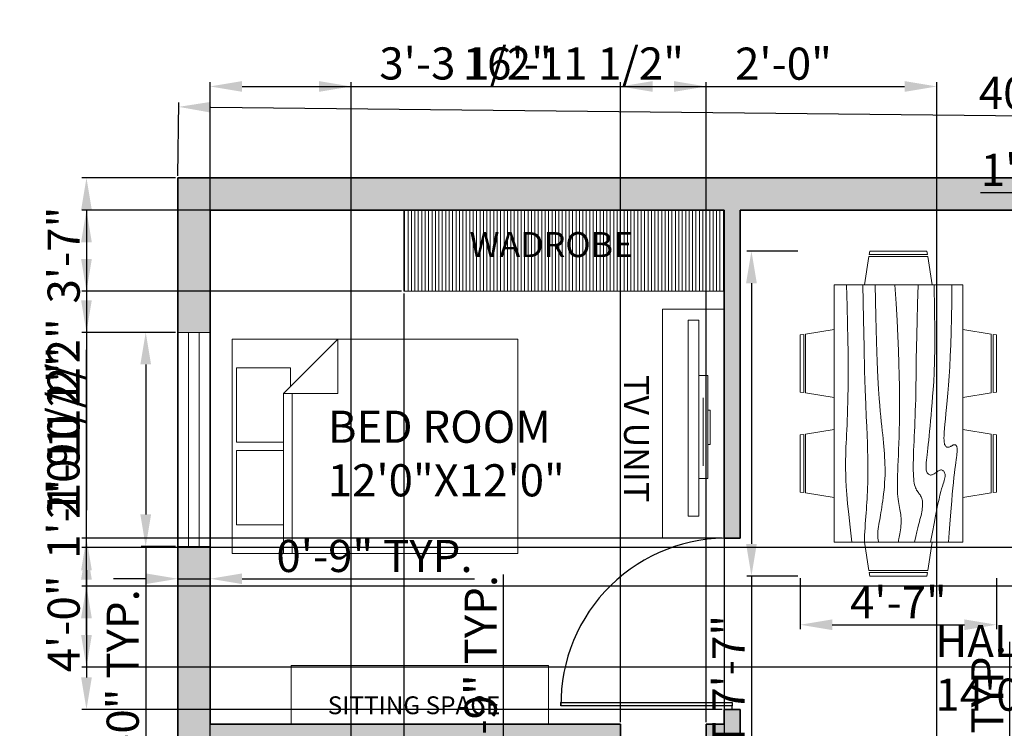
# Model space of a CAD drawing. Units: inches. Extents: x 33024 to 33675, y 11501 to 11939.
# Tile 2 of 3: x 33024 to 33299, y 11741 to 11939. Entities that reach past the tile are written whole.
import ezdxf

# ---------------------------------------------------------------- set-up
doc = ezdxf.new("R2010")
doc.units = ezdxf.units.IN
for name, color, linetype, lineweight in [('A-ANNO-DIMS', 2, 'Continuous', 18), ('A-ANNO-TEXT', 7, 'Continuous', 18), ('A-AREA-IDEN', 7, 'Continuous', 18), ('A-DOOR', 4, 'Continuous', 25), ('A-FURN', 8, 'Continuous', 18), ('A-FURN-FIXD', 8, 'Continuous', 18), ('A-FURN-PATT', 252, 'Continuous', 9), ('A-GLAZ', 4, 'Continuous', 18), ('A-WALL', 7, 'Continuous', 35)]:
    doc.layers.add(name, color=color, linetype=linetype, lineweight=lineweight)
doc.layers.add('A-WALL-PATT', color=242, linetype='Continuous', lineweight=13, true_color=0xcd2027)
doc.styles.get("Standard").update_dxf_attribs({"font": 'arial.ttf'})
doc.dimstyles.new('ISO-25', dxfattribs={"dimtxt": 9, "dimasz": 9, "dimexe": 1.25, "dimexo": 0.625, "dimtad": 1, "dimdec": 1, "dimrnd": 9, "dimlunit": 3, "dimtxsty": 'Standard', "dimcen": 2.5, "dimadec": 0, "dimazin": 0, "dimtfac": 1, "dimtdec": 1, "dimtmove": 0, "dimatfit": 3, "dimfxl": 1, "dimarcsym": 0})

# ---------------------------------------------------------------- blocks, each defined once
blk = doc.blocks.new('Bed - Queen')
for p, q in [((0, -80.00003), (0, 0)), ((0, 0), (59.99999, 0)), ((59.99999, 0), (59.99999, -80.00003)), ((7.99999, -1.2), (28.79998, -1.2)), ((7.99999, -14.4), (7.99999, -1.2)), ((28.79998, -1.2), (28.79998, -14.4)), ((31.19999, -1.2), (51.99999, -1.2)), ((31.19999, -14.4), (31.19999, -1.2)), ((51.99999, -1.2), (51.99999, -16.4)), ((0, -14.4), (44.8, -14.4)), ((59.99999, -29.6), (44.8, -14.4)), ((44.8, -14.4), (44.8, -29.6)), ((51.99999, -16.4), (46.79936, -16.4)), ((44.8, -16.8), (0, -16.8)), ((44.8, -29.6), (59.99999, -29.6)), ((59.99999, -80.00003), (0, -80.00003))]:
    blk.add_line(p, q)
blk = doc.blocks.new('Dining Set - 36 x 72 in.')
for p, q in [((-22.2343, 26.00059), (-23.4847, 17.99762)), ((-22.2304, 26), (-5.7608, 26)), ((-22, 27.5), (-22.1562, 26.50042)), ((-5.8416, 26.5), (-22.1534, 26.5)), ((-22, 27.5), (-6, 27.5)), ((-5.8437, 26.49966), (-6, 27.5)), ((-4.5152, 17.99762), (-5.7655, 25.99926)), ((5.7657, 26.00059), (4.5153, 17.99762)), ((5.7696, 26), (22.2392, 26)), ((6, 27.5), (5.8438, 26.50042)), ((22.1584, 26.5), (5.8466, 26.5)), ((6, 27.5), (22, 27.5)), ((22.1563, 26.49966), (22, 27.5)), ((23.4848, 17.99762), (22.2345, 25.99926)), ((36, 18), (-36, 18)), ((-36, 18), (-36, -18)), ((36, -18), (36, 18)), ((-44.0006, 8.23428), (-35.9976, 9.48474)), ((44.0006, 8.23428), (35.9976, 9.48474)), ((-45.5, 8), (-44.5004, 8.15617)), ((-45.5, 8), (-45.5, -8)), ((-44.5, -8.15843), (-44.5, 8.15338)), ((-44, 8.23041), (-44, -8.23915)), ((44, 8.23041), (44, -8.23915)), ((44.5, -8.15843), (44.5, 8.15338)), ((45.5, 8), (44.5005, 8.15617)), ((45.5, 8), (45.5, -8)), ((-44.4997, -8.15631), (-45.5, -8)), ((-35.9976, -9.48476), (-43.9993, -8.2345)), ((35.9976, -9.48476), (43.9993, -8.2345)), ((44.4997, -8.15631), (45.5, -8)), ((-36, -18), (36, -18)), ((-22.2343, -26.0006), (-23.4847, -17.99762)), ((-4.5152, -17.99762), (-5.7655, -25.99928)), ((5.7657, -26.0006), (4.5153, -17.99762)), ((23.4848, -17.99762), (22.2345, -25.99928)), ((-22.2304, -26), (-5.7608, -26)), ((-22, -27.5), (-22.1562, -26.50044)), ((-5.8416, -26.5), (-22.1534, -26.5)), ((-22, -27.5), (-6, -27.5)), ((-5.8437, -26.49967), (-6, -27.5)), ((5.7696, -26), (22.2392, -26)), ((6, -27.5), (5.8438, -26.50044)), ((22.1584, -26.5), (5.8466, -26.5)), ((6, -27.5), (22, -27.5)), ((22.1563, -26.49967), (22, -27.5))]:
    blk.add_line(p, q)
for points in [[(-36, 15), (-31.1772, 14.97754), (-26.8079, 14.91406), (-22.8538, 14.81543), (-19.276, 14.6875), (-16.0362, 14.53613), (-13.0957, 14.36718), (-10.4159, 14.18652), (-7.9583, 14), (-5.6904, 13.81315), (-3.6035, 13.63021), (-1.6954, 13.45508), (0.0365, 13.29166), (1.5945, 13.14388), (2.9811, 13.01562), (4.1988, 12.9108), (5.25, 12.83333), (6.1393, 12.78613), (6.8802, 12.76823), (7.4883, 12.77767), (7.9792, 12.8125), (8.3685, 12.87077), (8.6719, 12.95052), (8.9049, 13.0498), (9.0833, 13.16666), (9.2205, 13.29899), (9.3216, 13.44401), (9.3895, 13.59879), (9.4271, 13.76041), (9.4373, 13.92594), (9.4232, 14.09245), (9.3875, 14.257), (9.3333, 14.41666), (9.2638, 14.56917), (9.1836, 14.71484), (9.0975, 14.85465), (9.0104, 14.98958), (8.9272, 15.1206), (8.8529, 15.2487), (8.7922, 15.37483), (8.75, 15.5), (8.7305, 15.62467), (8.7344, 15.74739), (8.7617, 15.86621), (8.8125, 15.97916), (8.8867, 16.08431), (8.9844, 16.17968), (9.1055, 16.26334), (9.25, 16.33333), (9.4189, 16.38802), (9.6172, 16.42708), (9.8506, 16.45052), (10.125, 16.45833), (10.4463, 16.45052), (10.8203, 16.42708), (11.2529, 16.38802), (11.75, 16.33333), (12.3184, 16.26318), (12.9694, 16.17838), (13.7151, 16.07991), (14.5677, 15.96875), (15.5395, 15.84586), (16.6426, 15.71224), (17.8893, 15.56884), (19.2917, 15.41666), (20.859, 15.25667), (22.5879, 15.08984), (24.4721, 14.91715), (26.5052, 14.73958), (28.6809, 14.5581), (30.9929, 14.3737), (33.4347, 14.18733), (36, 14)], [(-36, 10), (-28.9766, 10.14274), (-23.1725, 10.20442), (-18.4241, 10.19775), (-14.5677, 10.13541), (-11.4399, 10.03011), (-8.877, 9.89453), (-6.7154, 9.74137), (-4.7917, 9.58333), (-2.9698, 9.43082), (-1.2246, 9.28515), (0.4415, 9.14534), (2.026, 9.01041), (3.5266, 8.87939), (4.9408, 8.7513), (6.266, 8.62516), (7.5, 8.5), (8.6411, 8.37549), (9.6914, 8.2539), (10.6538, 8.13818), (11.5312, 8.03125), (12.3267, 7.93603), (13.043, 7.85547), (13.6831, 7.79248), (14.25, 7.75), (14.7471, 7.7303), (15.1797, 7.73307), (15.5537, 7.75732), (15.875, 7.80208), (16.1494, 7.86637), (16.3828, 7.94922), (16.5811, 8.04964), (16.75, 8.16666), (16.8944, 8.29915), (17.0143, 8.44531), (17.1089, 8.60319), (17.1771, 8.77083), (17.218, 8.94629), (17.2305, 9.1276), (17.2137, 9.31282), (17.1667, 9.5), (17.0895, 9.6875), (16.987, 9.875), (16.8649, 10.0625), (16.7292, 10.25), (16.5856, 10.4375), (16.4401, 10.625), (16.2985, 10.8125), (16.1667, 11), (16.05, 11.18733), (15.9518, 11.3737), (15.8752, 11.5581), (15.8229, 11.73958), (15.798, 11.91715), (15.8034, 12.08984), (15.842, 12.25667), (15.9167, 12.41666), (16.0295, 12.56836), (16.1784, 12.70833), (16.3605, 12.83268), (16.5729, 12.9375), (16.8127, 13.01888), (17.0768, 13.07291), (17.3625, 13.0957), (17.6667, 13.08333), (17.9894, 13.03312), (18.3418, 12.94726), (18.7382, 12.82918), (19.1927, 12.68229), (19.7195, 12.51001), (20.3327, 12.31575), (21.0465, 12.10294), (21.875, 11.875), (22.8357, 11.63354), (23.959, 11.37304), (25.2786, 11.08618), (26.8282, 10.76562), (28.6414, 10.40405), (30.752, 9.99414), (33.1936, 9.52856), (36, 9)], [(-36, 5.5), (-30.7157, 5.3348), (-26.069, 5.20963), (-21.9946, 5.11767), (-18.4271, 5.05208), (-15.3009, 5.00602), (-12.5508, 4.97265), (-10.1112, 4.94515), (-7.9167, 4.91666), (-5.909, 4.88167), (-4.0586, 4.83984), (-2.3429, 4.79215), (-0.7396, 4.73958), (0.7739, 4.6831), (2.22, 4.6237), (3.6213, 4.56233), (5, 4.5), (6.373, 4.43782), (7.7344, 4.3776), (9.0723, 4.32129), (10.375, 4.27083), (11.6309, 4.22819), (12.8281, 4.19531), (13.9551, 4.17415), (15, 4.16666), (15.954, 4.17448), (16.819, 4.19791), (17.6001, 4.23698), (18.3021, 4.29166), (18.9299, 4.36198), (19.4883, 4.44791), (19.9823, 4.54948), (20.4167, 4.66666), (20.7969, 4.79899), (21.1302, 4.94401), (21.4245, 5.09879), (21.6875, 5.26041), (21.9271, 5.42594), (22.1511, 5.59245), (22.3672, 5.757), (22.5834, 5.91666), (22.8065, 6.06868), (23.0404, 6.21093), (23.2879, 6.34147), (23.5521, 6.45833), (23.8358, 6.55957), (24.142, 6.64323), (24.4735, 6.70735), (24.8334, 6.75), (25.2235, 6.76969), (25.642, 6.76692), (26.0858, 6.74267), (26.5521, 6.69791), (27.0379, 6.63362), (27.5404, 6.55078), (28.0565, 6.45036), (28.5834, 6.33333), (29.1242, 6.19987), (29.7071, 6.04687), (30.3661, 5.87044), (31.1354, 5.66666), (32.0493, 5.43164), (33.142, 5.16146), (34.4475, 4.85221), (36, 4.5)], [(-36, -1), (-30.7915, -0.6591), (-26.0195, -0.38216), (-21.6519, -0.16284), (-17.6563, 0.00521), (-14.0005, 0.12833), (-10.6523, 0.21289), (-7.5796, 0.26522), (-4.75, 0.29166), (-2.134, 0.29793), (0.2878, 0.28711), (2.5317, 0.26163), (4.6146, 0.22396), (6.5529, 0.17651), (8.3633, 0.12174), (10.0623, 0.06209), (11.6667, 0), (13.1899, -0.06201), (14.6341, -0.1211), (15.9982, -0.17432), (17.2813, -0.21875), (18.4823, -0.25147), (19.6003, -0.26953), (20.6343, -0.27002), (21.5834, -0.25), (22.4481, -0.20768), (23.2357, -0.14584), (23.9549, -0.06836), (24.6146, 0.02083), (25.2235, 0.11784), (25.7904, 0.21875), (26.3241, 0.31966), (26.8334, 0.41666), (27.3265, 0.50618), (27.8099, 0.58593), (28.2894, 0.65397), (28.7709, 0.70833), (29.2601, 0.74707), (29.763, 0.76823), (30.2855, 0.76985), (30.8334, 0.75), (31.4088, 0.70784), (31.9994, 0.64713), (32.589, 0.57275), (33.1615, 0.48958), (33.7008, 0.4025), (34.1908, 0.3164), (34.6153, 0.23616), (34.9584, 0.16666), (35.2099, 0.11165), (35.3848, 0.07031), (35.504, 0.04069), (35.5886, 0.02083), (35.6594, 0.00879), (35.7377, 0.0026), (35.8442, 0.00032), (36, 0)], [(-36, -6.5), (-27.1843, -6.31267), (-20.084, -6.1263), (-14.469, -5.9419), (-10.1094, -5.76042), (-6.7752, -5.58285), (-4.2363, -5.41016), (-2.2629, -5.24333), (-0.625, -5.08334), (0.8708, -4.93099), (2.2715, -4.78646), (3.5872, -4.64974), (4.8281, -4.52084), (6.0046, -4.39974), (7.127, -4.28646), (8.2053, -4.18099), (9.25, -4.08334), (10.2705, -3.99382), (11.2734, -3.91407), (12.2647, -3.84603), (13.25, -3.79167), (14.2354, -3.75293), (15.2266, -3.73177), (16.2295, -3.73015), (17.25, -3.75), (18.2912, -3.79248), (19.3451, -3.85547), (20.4009, -3.93604), (21.4479, -4.03125), (22.4754, -4.13819), (23.4727, -4.25391), (24.4289, -4.37549), (25.3334, -4.5), (26.1785, -4.62492), (26.9694, -4.74935), (27.7145, -4.87281), (28.4219, -4.99479), (29.1, -5.11483), (29.7572, -5.23242), (30.4016, -5.34709), (31.0417, -5.45834), (31.6837, -5.56437), (32.3262, -5.65821), (32.9658, -5.73153), (33.599, -5.77604), (34.2224, -5.78345), (34.8327, -5.74545), (35.4264, -5.65373), (36, -5.5)], [(-36, -10), (-26.4022, -9.81299), (-18.4675, -9.62891), (-11.9839, -9.45069), (-6.7396, -9.28125), (-2.5226, -9.12354), (0.8789, -8.98047), (3.6769, -8.85498), (6.0833, -8.75), (8.2767, -8.66765), (10.3021, -8.60677), (12.1712, -8.56543), (13.8958, -8.54167), (15.4876, -8.53353), (16.9583, -8.53907), (18.3197, -8.55632), (19.5834, -8.58334), (20.7616, -8.61841), (21.8685, -8.66081), (22.9188, -8.71004), (23.9271, -8.76563), (24.9081, -8.82707), (25.8763, -8.89388), (26.8465, -8.96558), (27.8334, -9.04167), (28.8474, -9.12118), (29.8828, -9.20117), (30.93, -9.27824), (31.9792, -9.34896), (33.0205, -9.40991), (34.0443, -9.45768), (35.0407, -9.48885), (36, -9.5)], [(-36, -14.5), (-30.0881, -14.33513), (-25.0332, -14.21224), (-20.7312, -14.12647), (-17.0781, -14.07292), (-13.97, -14.04671), (-11.3027, -14.04297), (-8.9724, -14.05681), (-6.875, -14.08334), (-4.9224, -14.11833), (-3.0905, -14.16016), (-1.3709, -14.20785), (0.2448, -14.26042), (1.7647, -14.3169), (3.1973, -14.3763), (4.5507, -14.43767), (5.8333, -14.5), (7.0554, -14.5621), (8.235, -14.62175), (9.3922, -14.67652), (10.5469, -14.72396), (11.7192, -14.76164), (12.929, -14.78711), (14.1965, -14.79794), (15.5417, -14.79167), (16.9933, -14.76424), (18.6152, -14.70508), (20.4804, -14.60197), (22.6615, -14.44271), (25.2312, -14.21509), (28.2624, -13.9069), (31.8277, -13.50594), (36, -13)]]:
    blk.add_lwpolyline(points)
blk = doc.blocks.new('*D8')
at = {"layer": 'A-ANNO-DIMS', "color": 0, "lineweight": -2, "transparency": 16777216}
for p, q in [((33068.04, 11895.8), (33068.26, 11916.32)), ((33077.25, 11914.97), (33541.21, 11909.99)), ((33550.01, 11890.62), (33550.23, 11911.14))]:
    blk.add_line(p, q, dxfattribs=at)
at = {"layer": 'A-ANNO-DIMS', "color": 0, "transparency": 16777216}
for points in [[(33077.26, 11916.47), (33077.23, 11913.47), (33068.25, 11915.07)], [(33541.23, 11911.49), (33541.2, 11908.49), (33550.21, 11909.89)]]:
    blk.add_solid(points, dxfattribs=at)
at = {"layer": 'Defpoints', "color": 0, "transparency": 16777216}
for p in [(33550.21, 11909.89), (33068.03, 11895.18), (33550, 11890)]:
    blk.add_point(p, dxfattribs=at)
at = {"layer": 'A-ANNO-DIMS', "color": 0, "transparency": 16777216, "insert": (33309.29, 11917.7), "char_height": 9, "attachment_point": 5, "rotation": 359.3847}
blk.add_mtext('40\'-6"', dxfattribs=at)
blk = doc.blocks.new('TV-CONSOLE-64')
for p, q in [((-17.33, 64.14), (-17.33, 0)), ((-7.13, 45.53), (-7.13, 45.53)), ((-7.13, 45.53), (-4.58, 45.53)), ((-4.58, 45.53), (-4.58, 16.72)), ((-5.92, 39.3), (-5.92, 20.26)), ((-4.58, 35.87), (-3.95, 35.87)), ((-3.95, 35.87), (-3.95, 26.18)), ((-3.95, 26.18), (-4.58, 26.18)), ((-4.58, 16.72), (-7.13, 16.72))]:
    blk.add_line(p, q)
blk.add_lwpolyline([(-17.33, 64.14), (0, 64.14), (0, 0), (-17.33, 0)])
blk.add_lwpolyline([(-10.08, 61), (-7.13, 61), (-7.13, 6.14), (-10.08, 6.14)], close=True)
blk = doc.blocks.new('WIN-60X9')
for p, q in [((0, 9), (0, 0)), ((60, 9), (60, 0)), ((60, 6), (0, 6)), ((60, 3), (0, 3))]:
    blk.add_line(p, q)
blk = doc.blocks.new('*D12')
at = {"layer": 'A-ANNO-DIMS', "color": 0, "lineweight": -2, "transparency": 16777216}
for p, q in [((33067.41, 11851.93), (33057.78, 11851.93)), ((33059.03, 11842.93), (33059.03, 11800.93)), ((33067.41, 11791.93), (33057.78, 11791.93)), ((33059.03, 11791.93), (33059.03, 11667.8))]:
    blk.add_line(p, q, dxfattribs=at)
at = {"layer": 'A-ANNO-DIMS', "color": 0, "transparency": 16777216}
for points in [[(33057.53, 11842.93), (33060.53, 11842.93), (33059.03, 11851.93)], [(33057.53, 11800.93), (33060.53, 11800.93), (33059.03, 11791.93)]]:
    blk.add_solid(points, dxfattribs=at)
at = {"layer": 'Defpoints', "color": 0, "transparency": 16777216}
for p in [(33068.03, 11851.93), (33059.03, 11791.93), (33068.03, 11791.93)]:
    blk.add_point(p, dxfattribs=at)
at = {"layer": 'A-ANNO-DIMS', "color": 0, "transparency": 16777216, "insert": (33053.75, 11725.37), "char_height": 9, "attachment_point": 5, "rotation": 90}
blk.add_mtext('WINDOW 5\'-0" TYP.', dxfattribs=at)
blk = doc.blocks.new('*D13')
at = {"layer": 'A-ANNO-DIMS', "color": 0, "lineweight": -2, "transparency": 16777216}
for p, q in [((33068.03, 11791.31), (33068.03, 11781.68)), ((33077.03, 11791.31), (33077.03, 11781.68)), ((33059.03, 11782.93), (33050.03, 11782.93)), ((33068.03, 11782.93), (33077.03, 11782.93)), ((33086.03, 11782.93), (33151.14, 11782.93))]:
    blk.add_line(p, q, dxfattribs=at)
at = {"layer": 'A-ANNO-DIMS', "color": 0, "transparency": 16777216}
for points in [[(33059.03, 11784.43), (33059.03, 11781.43), (33068.03, 11782.93)], [(33086.03, 11784.43), (33086.03, 11781.43), (33077.03, 11782.93)]]:
    blk.add_solid(points, dxfattribs=at)
at = {"layer": 'Defpoints', "color": 0, "transparency": 16777216}
for p in [(33068.03, 11791.93), (33077.03, 11791.93), (33077.03, 11782.93)]:
    blk.add_point(p, dxfattribs=at)
at = {"layer": 'A-ANNO-DIMS', "color": 0, "transparency": 16777216, "insert": (33123.09, 11788.15), "char_height": 9, "attachment_point": 5}
blk.add_mtext('0\'-9" TYP.', dxfattribs=at)
blk = doc.blocks.new('*D15')
at = {"layer": 'A-ANNO-DIMS', "color": 0, "lineweight": -2, "transparency": 16777216}
for p, q in [((33387.03, 11881.98), (33387.03, 11892.22)), ((33404.36, 11881.98), (33404.36, 11892.22)), ((33378.03, 11890.97), (33292.8, 11890.97)), ((33404.36, 11890.97), (33387.03, 11890.97)), ((33413.36, 11890.97), (33422.36, 11890.97))]:
    blk.add_line(p, q, dxfattribs=at)
at = {"layer": 'A-ANNO-DIMS', "color": 0, "transparency": 16777216}
for points in [[(33378.03, 11892.47), (33378.03, 11889.47), (33387.03, 11890.97)], [(33413.36, 11892.47), (33413.36, 11889.47), (33404.36, 11890.97)]]:
    blk.add_solid(points, dxfattribs=at)
at = {"layer": 'Defpoints', "color": 0, "transparency": 16777216}
for p in [(33387.03, 11890.97), (33387.03, 11881.35), (33404.36, 11881.35)]:
    blk.add_point(p, dxfattribs=at)
at = {"layer": 'A-ANNO-DIMS', "color": 0, "transparency": 16777216, "insert": (33330.92, 11896.25), "char_height": 9, "attachment_point": 5}
blk.add_mtext('1\'-5 1/2" TYP.', dxfattribs=at)
blk = doc.blocks.new('*D16')
at = {"layer": 'A-ANNO-DIMS', "color": 0, "lineweight": -2, "transparency": 16777216}
for p, q in [((33121.2, 11724.86), (33031.28, 11724.86)), ((33121.2, 11720.53), (33121.2, 11726.11)), ((33145.25, 11724.86), (33130.2, 11724.86)), ((33154.25, 11720.53), (33154.25, 11726.11))]:
    blk.add_line(p, q, dxfattribs=at)
at = {"layer": 'A-ANNO-DIMS', "color": 0, "transparency": 16777216}
for points in [[(33130.2, 11726.36), (33130.2, 11723.36), (33121.2, 11724.86)], [(33145.25, 11726.36), (33145.25, 11723.36), (33154.25, 11724.86)]]:
    blk.add_solid(points, dxfattribs=at)
at = {"layer": 'Defpoints', "color": 0, "transparency": 16777216}
for p in [(33121.2, 11724.86), (33121.2, 11719.9), (33154.25, 11719.9)]:
    blk.add_point(p, dxfattribs=at)
at = {"layer": 'A-ANNO-DIMS', "color": 0, "transparency": 16777216, "insert": (33071.74, 11730.14), "char_height": 9, "attachment_point": 5}
blk.add_mtext('WC 2\'-9" TYP.', dxfattribs=at)
blk = doc.blocks.new('*D17')
at = {"layer": 'A-ANNO-DIMS', "color": 0, "lineweight": -2, "transparency": 16777216}
for p, q in [((33159.2, 11719.9), (33159.2, 11784.16)), ((33154.87, 11719.9), (33160.45, 11719.9)), ((33159.2, 11707.9), (33159.2, 11710.9)), ((33154.87, 11698.9), (33160.45, 11698.9))]:
    blk.add_line(p, q, dxfattribs=at)
at = {"layer": 'A-ANNO-DIMS', "color": 0, "transparency": 16777216}
for points in [[(33157.7, 11710.9), (33160.7, 11710.9), (33159.2, 11719.9)], [(33157.7, 11707.9), (33160.7, 11707.9), (33159.2, 11698.9)]]:
    blk.add_solid(points, dxfattribs=at)
at = {"layer": 'Defpoints', "color": 0, "transparency": 16777216}
for p in [(33154.25, 11719.9), (33159.2, 11719.9), (33154.25, 11698.9)]:
    blk.add_point(p, dxfattribs=at)
at = {"layer": 'A-ANNO-DIMS', "color": 0, "transparency": 16777216, "insert": (33153.98, 11756.53), "char_height": 9, "attachment_point": 5, "rotation": 90}
blk.add_mtext('1\'-9" TYP.', dxfattribs=at)
blk = doc.blocks.new('*D23')
at = {"layer": 'A-ANNO-DIMS', "color": 0, "lineweight": -2, "transparency": 16777216}
for p, q in [((33301, 11700), (33301, 11765.26)), ((33309.38, 11700), (33299.75, 11700)), ((33301, 11678), (33301, 11691)), ((33309.38, 11669), (33299.75, 11669))]:
    blk.add_line(p, q, dxfattribs=at)
at = {"layer": 'A-ANNO-DIMS', "color": 0, "transparency": 16777216}
for points in [[(33299.5, 11691), (33302.5, 11691), (33301, 11700)], [(33299.5, 11678), (33302.5, 11678), (33301, 11669)]]:
    blk.add_solid(points, dxfattribs=at)
at = {"layer": 'Defpoints', "color": 0, "transparency": 16777216}
for p in [(33301, 11700), (33310, 11700), (33310, 11669)]:
    blk.add_point(p, dxfattribs=at)
at = {"layer": 'A-ANNO-DIMS', "color": 0, "transparency": 16777216, "insert": (33295.85, 11737.13), "char_height": 9, "attachment_point": 5, "rotation": 90}
blk.add_mtext('2\'-7" TYP.', dxfattribs=at)
blk = doc.blocks.new('*D28')
at = {"layer": 'A-ANNO-DIMS', "color": 0, "lineweight": -2, "transparency": 16777216}
for p, q in [((33241.67, 11874.7), (33227.4, 11874.7)), ((33228.65, 11865.7), (33228.65, 11792.7)), ((33241.67, 11783.7), (33227.4, 11783.7)), ((33228.65, 11783.7), (33228.65, 11674.53))]:
    blk.add_line(p, q, dxfattribs=at)
at = {"layer": 'A-ANNO-DIMS', "color": 0, "transparency": 16777216}
for points in [[(33227.15, 11865.7), (33230.15, 11865.7), (33228.65, 11874.7)], [(33227.15, 11792.7), (33230.15, 11792.7), (33228.65, 11783.7)]]:
    blk.add_solid(points, dxfattribs=at)
at = {"layer": 'Defpoints', "color": 0, "transparency": 16777216}
for p in [(33242.3, 11874.7), (33228.65, 11783.7), (33242.3, 11783.7)]:
    blk.add_point(p, dxfattribs=at)
at = {"layer": 'A-ANNO-DIMS', "color": 0, "transparency": 16777216, "insert": (33223.37, 11724.62), "char_height": 9, "attachment_point": 5, "rotation": 90}
blk.add_mtext('DINING SET 7\'-7"', dxfattribs=at)
blk = doc.blocks.new('*D29')
at = {"layer": 'A-ANNO-DIMS', "color": 0, "lineweight": -2, "transparency": 16777216}
for p, q in [((33242.298915, 11783.0767), (33242.298915, 11768.8017)), ((33297.298915, 11783.0767), (33297.298915, 11768.8017)), ((33251.298915, 11770.0517), (33288.298915, 11770.0517))]:
    blk.add_line(p, q, dxfattribs=at)
at = {"layer": 'A-ANNO-DIMS', "color": 0, "transparency": 16777216}
for points in [[(33251.298915, 11771.5517), (33251.298915, 11768.5517), (33242.298915, 11770.0517)], [(33288.298915, 11771.5517), (33288.298915, 11768.5517), (33297.298915, 11770.0517)]]:
    blk.add_solid(points, dxfattribs=at)
at = {"layer": 'Defpoints', "color": 0, "transparency": 16777216}
for p in [(33242.298915, 11783.7017), (33297.298915, 11783.7017), (33297.298915, 11770.0517)]:
    blk.add_point(p, dxfattribs=at)
at = {"layer": 'A-ANNO-DIMS', "color": 0, "transparency": 16777216, "insert": (33269.798915, 11775.1767), "char_height": 9, "attachment_point": 5}
blk.add_mtext('4\'-7"', dxfattribs=at)
blk = doc.blocks.new('*D30')
at = {"layer": 'A-ANNO-DIMS', "color": 0, "lineweight": -2, "transparency": 16777216}
for p, q in [((33067.41, 11895.18), (33041.18, 11895.18)), ((33042.43, 11886.18), (33042.43, 11860.93)), ((33067.41, 11851.93), (33041.18, 11851.93))]:
    blk.add_line(p, q, dxfattribs=at)
at = {"layer": 'A-ANNO-DIMS', "color": 0, "transparency": 16777216}
for points in [[(33040.93, 11886.18), (33043.93, 11886.18), (33042.43, 11895.18)], [(33040.93, 11860.93), (33043.93, 11860.93), (33042.43, 11851.93)]]:
    blk.add_solid(points, dxfattribs=at)
at = {"layer": 'Defpoints', "color": 0, "transparency": 16777216}
for p in [(33068.03, 11895.18), (33042.43, 11851.93), (33068.03, 11851.93)]:
    blk.add_point(p, dxfattribs=at)
at = {"layer": 'A-ANNO-DIMS', "color": 0, "transparency": 16777216, "insert": (33037.21, 11873.56), "char_height": 9, "attachment_point": 5, "rotation": 90}
blk.add_mtext('3\'-7"', dxfattribs=at)
blk = doc.blocks.new('*D31')
at = {"layer": 'A-ANNO-DIMS', "color": 0, "lineweight": -2, "transparency": 16777216}
for p, q in [((33042.43, 11791.72), (33042.43, 11847.01)), ((33538.41, 11791.72), (33041.18, 11791.72)), ((33042.43, 11767.18), (33042.43, 11782.72)), ((33538.41, 11758.18), (33041.18, 11758.18))]:
    blk.add_line(p, q, dxfattribs=at)
at = {"layer": 'A-ANNO-DIMS', "color": 0, "transparency": 16777216}
for points in [[(33040.93, 11782.72), (33043.93, 11782.72), (33042.43, 11791.72)], [(33040.93, 11767.18), (33043.93, 11767.18), (33042.43, 11758.18)]]:
    blk.add_solid(points, dxfattribs=at)
at = {"layer": 'Defpoints', "color": 0, "transparency": 16777216}
for p in [(33042.43, 11791.72), (33539.03, 11791.72), (33539.03, 11758.18)]:
    blk.add_point(p, dxfattribs=at)
at = {"layer": 'A-ANNO-DIMS', "color": 0, "transparency": 16777216, "insert": (33037.15, 11823.87), "char_height": 9, "attachment_point": 5, "rotation": 90}
blk.add_mtext('2\'-9 1/2"', dxfattribs=at)
blk = doc.blocks.new('*D35')
at = {"layer": 'A-ANNO-DIMS', "color": 0, "lineweight": -2, "transparency": 16777216}
for p, q in [((33220.41, 11794.3), (33041.18, 11794.3)), ((33042.43, 11785.3), (33042.43, 11755.3)), ((33220.41, 11746.3), (33041.18, 11746.3))]:
    blk.add_line(p, q, dxfattribs=at)
at = {"layer": 'A-ANNO-DIMS', "color": 0, "transparency": 16777216}
for points in [[(33040.93, 11785.3), (33043.93, 11785.3), (33042.43, 11794.3)], [(33040.93, 11755.3), (33043.93, 11755.3), (33042.43, 11746.3)]]:
    blk.add_solid(points, dxfattribs=at)
at = {"layer": 'Defpoints', "color": 0, "transparency": 16777216}
for p in [(33221.03, 11794.3), (33042.43, 11746.3), (33221.03, 11746.3)]:
    blk.add_point(p, dxfattribs=at)
at = {"layer": 'A-ANNO-DIMS', "color": 0, "transparency": 16777216, "insert": (33037.21, 11770.3), "char_height": 9, "attachment_point": 5, "rotation": 90}
blk.add_mtext('4\'-0"', dxfattribs=at)
blk = doc.blocks.new('*D37')
at = {"layer": 'A-ANNO-DIMS', "color": 0, "lineweight": -2, "transparency": 16777216}
for p, q in [((33191.96, 11742.8), (33191.96, 11922.03)), ((33200.96, 11920.78), (33206.96, 11920.78)), ((33215.96, 11742.8), (33215.96, 11922.03)), ((33215.96, 11920.78), (33250.28, 11920.78))]:
    blk.add_line(p, q, dxfattribs=at)
at = {"layer": 'A-ANNO-DIMS', "color": 0, "transparency": 16777216}
for points in [[(33200.96, 11922.28), (33200.96, 11919.28), (33191.96, 11920.78)], [(33206.96, 11922.28), (33206.96, 11919.28), (33215.96, 11920.78)]]:
    blk.add_solid(points, dxfattribs=at)
at = {"layer": 'Defpoints', "color": 0, "transparency": 16777216}
for p in [(33215.96, 11920.78), (33191.96, 11742.18), (33215.96, 11742.18)]:
    blk.add_point(p, dxfattribs=at)
at = {"layer": 'A-ANNO-DIMS', "color": 0, "transparency": 16777216, "insert": (33237.62, 11926), "char_height": 9, "attachment_point": 5}
blk.add_mtext('2\'-0"', dxfattribs=at)
blk = doc.blocks.new('*D40')
at = {"layer": 'A-ANNO-DIMS', "color": 0, "lineweight": -2, "transparency": 16777216}
for p, q in [((33077.03, 11535.8), (33077.03, 11922.03)), ((33086.03, 11920.78), (33271.53, 11920.78)), ((33280.53, 11535.8), (33280.53, 11922.03))]:
    blk.add_line(p, q, dxfattribs=at)
at = {"layer": 'A-ANNO-DIMS', "color": 0, "transparency": 16777216}
for points in [[(33086.03, 11922.28), (33086.03, 11919.28), (33077.03, 11920.78)], [(33271.53, 11922.28), (33271.53, 11919.28), (33280.53, 11920.78)]]:
    blk.add_solid(points, dxfattribs=at)
at = {"layer": 'Defpoints', "color": 0, "transparency": 16777216}
for p in [(33280.53, 11920.78), (33077.03, 11535.18), (33280.53, 11535.18)]:
    blk.add_point(p, dxfattribs=at)
at = {"layer": 'A-ANNO-DIMS', "color": 0, "transparency": 16777216, "insert": (33178.78, 11926.05), "char_height": 9, "attachment_point": 5}
blk.add_mtext('16\'-11 1/2"', dxfattribs=at)
blk = doc.blocks.new('*D43')
at = {"layer": 'A-ANNO-DIMS', "color": 0, "lineweight": -2, "transparency": 16777216}
for p, q in [((33130.68, 11886.18), (33041.18, 11886.18)), ((33042.43, 11877.18), (33042.43, 11872.46)), ((33130.68, 11863.46), (33041.18, 11863.46)), ((33042.43, 11863.46), (33042.43, 11802.17))]:
    blk.add_line(p, q, dxfattribs=at)
at = {"layer": 'A-ANNO-DIMS', "color": 0, "transparency": 16777216}
for points in [[(33040.93, 11877.18), (33043.93, 11877.18), (33042.43, 11886.18)], [(33040.93, 11872.46), (33043.93, 11872.46), (33042.43, 11863.46)]]:
    blk.add_solid(points, dxfattribs=at)
at = {"layer": 'Defpoints', "color": 0, "transparency": 16777216}
for p in [(33131.3, 11886.18), (33042.43, 11863.46), (33131.3, 11863.46)]:
    blk.add_point(p, dxfattribs=at)
at = {"layer": 'A-ANNO-DIMS', "color": 0, "transparency": 16777216, "insert": (33037.15, 11828.31), "char_height": 9, "attachment_point": 5, "rotation": 90}
blk.add_mtext('1\'-10 1/2"', dxfattribs=at)
blk = doc.blocks.new('*D44')
at = {"layer": 'A-ANNO-DIMS', "color": 0, "lineweight": -2, "transparency": 16777216}
for p, q in [((33131.3, 11862.83), (33131.3, 11508.33)), ((33221.03, 11862.83), (33221.03, 11508.33)), ((33140.3, 11509.58), (33212.03, 11509.58))]:
    blk.add_line(p, q, dxfattribs=at)
at = {"layer": 'A-ANNO-DIMS', "color": 0, "transparency": 16777216}
for points in [[(33140.3, 11511.08), (33140.3, 11508.08), (33131.3, 11509.58)], [(33212.03, 11511.08), (33212.03, 11508.08), (33221.03, 11509.58)]]:
    blk.add_solid(points, dxfattribs=at)
at = {"layer": 'Defpoints', "color": 0, "transparency": 16777216}
for p in [(33131.3, 11863.46), (33221.03, 11863.46), (33221.03, 11509.58)]:
    blk.add_point(p, dxfattribs=at)
at = {"layer": 'A-ANNO-DIMS', "color": 0, "transparency": 16777216, "insert": (33176.17, 11514.85), "char_height": 9, "attachment_point": 5}
blk.add_mtext('7\'-5 1/2"', dxfattribs=at)
blk = doc.blocks.new('*D46')
at = {"layer": 'A-ANNO-DIMS', "color": 0, "lineweight": -2, "transparency": 16777216}
for p, q in [((33042.43, 11780.89), (33042.43, 11842.18)), ((33490.92, 11780.89), (33041.18, 11780.89)), ((33042.43, 11767.18), (33042.43, 11771.89)), ((33490.92, 11758.18), (33041.18, 11758.18))]:
    blk.add_line(p, q, dxfattribs=at)
at = {"layer": 'A-ANNO-DIMS', "color": 0, "transparency": 16777216}
for points in [[(33040.93, 11771.89), (33043.93, 11771.89), (33042.43, 11780.89)], [(33040.93, 11767.18), (33043.93, 11767.18), (33042.43, 11758.18)]]:
    blk.add_solid(points, dxfattribs=at)
at = {"layer": 'Defpoints', "color": 0, "transparency": 16777216}
for p in [(33042.43, 11780.89), (33491.54, 11780.89), (33491.54, 11758.18)]:
    blk.add_point(p, dxfattribs=at)
at = {"layer": 'A-ANNO-DIMS', "color": 0, "transparency": 16777216, "insert": (33037.15, 11816.04), "char_height": 9, "attachment_point": 5, "rotation": 90}
blk.add_mtext('1\'-10 1/2"', dxfattribs=at)
blk = doc.blocks.new('*D49')
at = {"layer": 'A-ANNO-DIMS', "color": 0, "lineweight": -2, "transparency": 16777216}
for p, q in [((33077.03, 11685.8), (33077.03, 11922.03)), ((33086.03, 11920.78), (33107.53, 11920.78)), ((33116.53, 11685.8), (33116.53, 11922.03)), ((33116.53, 11920.78), (33171.67, 11920.78))]:
    blk.add_line(p, q, dxfattribs=at)
at = {"layer": 'A-ANNO-DIMS', "color": 0, "transparency": 16777216}
for points in [[(33086.03, 11922.28), (33086.03, 11919.28), (33077.03, 11920.78)], [(33107.53, 11922.28), (33107.53, 11919.28), (33116.53, 11920.78)]]:
    blk.add_solid(points, dxfattribs=at)
at = {"layer": 'Defpoints', "color": 0, "transparency": 16777216}
for p in [(33116.53, 11920.78), (33077.03, 11685.18), (33116.53, 11685.18)]:
    blk.add_point(p, dxfattribs=at)
at = {"layer": 'A-ANNO-DIMS', "color": 0, "transparency": 16777216, "insert": (33148.6, 11926.06), "char_height": 9, "attachment_point": 5}
blk.add_mtext('3\'-3 1/2"', dxfattribs=at)

msp = doc.modelspace()

# ---------------------------------------------------------------- hatches: boundary and pattern name
at = {"layer": 'A-FURN-PATT'}
h = msp.add_hatch(dxfattribs=at)
h.set_pattern_fill('ANSI31', color=256, scale=0.3023622, angle=45, style=0)
h.paths.add_polyline_path([(33131.3, 11863.46), (33221.03, 11863.46), (33221.03, 11886.18), (33131.3, 11886.18)])
at = {"layer": 'A-WALL-PATT'}
h = msp.add_hatch(color=256, dxfattribs=at)
h.dxf.hatch_style = 1
h.paths.add_polyline_path([(33548.03, 11895.18), (33068.03, 11895.18), (33068.03, 11851.93), (33077.03, 11851.93), (33077.03, 11886.18), (33221.03, 11886.18), (33221.03, 11794.32, -0.012093), (33223.28, 11794.3), (33225.53, 11794.3), (33225.53, 11886.18), (33382.53, 11886.18), (33382.53, 11845.96, -0.043682), (33382.53, 11826.04), (33382.53, 11810.27), (33384.78, 11810.27, -0.005263), (33385.78, 11810.27), (33387.03, 11810.27), (33387.03, 11886.18), (33539.03, 11886.18), (33539.03, 11851.72), (33548.03, 11851.72)])
h.paths.add_polyline_path([(33077.03, 11791.93), (33068.03, 11791.93), (33068.03, 11535.18), (33077.03, 11535.18), (33077.03, 11544.18), (33077.03, 11737.68), (33116.53, 11737.68), (33116.53, 11685.18), (33221.03, 11685.18), (33221.03, 11617.18), (33228.7, 11617.18), (33228.7, 11626.18), (33225.53, 11626.18), (33225.53, 11746.3), (33221.03, 11746.3), (33221.03, 11742.18), (33215.96, 11742.18), (33215.96, 11737.68), (33221.03, 11737.68), (33221.03, 11689.68), (33121.03, 11689.68), (33121.03, 11737.68), (33179.96, 11737.68), (33191.96, 11737.68), (33191.96, 11738.93, -0.010637), (33191.96, 11739.93), (33191.96, 11742.18), (33179.96, 11742.18), (33077.03, 11742.18)])
h.paths.add_polyline_path([(33548.03, 11791.72), (33539.03, 11791.72), (33539.03, 11758.18), (33426.07, 11758.18), (33414.07, 11758.18), (33414.07, 11755.93, -0.023906), (33414.1, 11753.68), (33426.07, 11753.68), (33487.03, 11753.68), (33487.03, 11705.68), (33387.03, 11705.68), (33387.03, 11753.68), (33390.07, 11753.68), (33390.07, 11754.93), (33390.07, 11755.93), (33390.07, 11758.18), (33387.03, 11758.18), (33387.03, 11762.27), (33382.53, 11762.27), (33382.53, 11701.18), (33387.03, 11701.18), (33491.53, 11701.18), (33491.53, 11753.68), (33539.03, 11753.68), (33539.03, 11581.18), (33498.14, 11581.18), (33498.14, 11572.18), (33539.03, 11572.18), (33539.03, 11544.18), (33280.53, 11544.18), (33280.53, 11535.18), (33548.03, 11535.18)])
h.paths.add_polyline_path([(33391.53, 11626.18), (33391.53, 11626.18), (33391.53, 11665.18), (33382.53, 11665.18), (33382.53, 11626.18), (33358.03, 11626.18), (33358.03, 11617.18), (33382.53, 11617.18), (33382.53, 11572.18), (33387.03, 11572.18), (33438.14, 11572.18), (33438.14, 11581.18), (33391.53, 11581.18), (33391.53, 11614.89)], flags=17)

# ---------------------------------------------------------------- linework, layer by layer
at = {"layer": 'A-DOOR'}
for p, q in [((33175.28, 11747.3), (33175.28, 11748.3)), ((33175.28, 11748.3), (33223.28, 11748.3)), ((33223.28, 11747.3), (33175.28, 11747.3)), ((33223.28, 11748.3), (33223.28, 11747.3)), ((33223.28, 11746.3), (33223.28, 11747.3))]:
    msp.add_line(p, q, dxfattribs=at)
msp.add_arc((33221.8, 11747.8), 46.52, 88.178, 180.6158, dxfattribs=at)
at = {"layer": 'A-FURN-FIXD'}
for p, q in [((33131.3, 11863.46), (33131.3, 11886.18)), ((33221.03, 11863.46), (33131.3, 11863.46)), ((33099.75, 11742.18), (33099.75, 11758.66)), ((33099.75, 11758.66), (33171.77, 11758.66)), ((33171.77, 11758.66), (33171.77, 11742.18))]:
    msp.add_line(p, q, dxfattribs=at)
at = {"layer": 'A-WALL'}
for p, q in [((33548.03, 11895.18), (33068.03, 11895.18)), ((33068.03, 11895.18), (33068.03, 11535.18)), ((33077.03, 11886.18), (33077.03, 11742.18)), ((33221.03, 11886.18), (33077.03, 11886.18)), ((33221.03, 11886.18), (33221.03, 11794.3)), ((33225.53, 11886.18), (33225.53, 11794.3)), ((33382.53, 11886.18), (33225.53, 11886.18)), ((33221.03, 11794.3), (33225.53, 11794.3)), ((33221.03, 11746.3), (33225.53, 11746.3)), ((33221.03, 11746.3), (33221.03, 11742.18)), ((33225.53, 11746.3), (33225.53, 11626.18)), ((33179.96, 11742.18), (33077.03, 11742.18)), ((33179.96, 11742.18), (33191.96, 11742.18)), ((33191.96, 11742.18), (33191.96, 11737.68)), ((33221.03, 11742.18), (33215.96, 11742.18)), ((33215.96, 11742.18), (33215.96, 11737.68))]:
    msp.add_line(p, q, dxfattribs=at)

# ---------------------------------------------------------------- block references
at = {"layer": 'A-FURN'}
for name, p, rotation in [('Dining Set - 36 x 72 in.', (33269.8, 11829.2), 270), ('Bed - Queen', (33083.2, 11790), 89.99999999999999)]:
    msp.add_blockref(name, p, dxfattribs=dict(at, rotation=rotation))
at = {"layer": 'A-FURN-FIXD'}
msp.add_blockref('TV-CONSOLE-64', (33221.03, 11794.3), dxfattribs=at)
at = {"layer": 'A-GLAZ', "rotation": 269.9999999999987}
msp.add_blockref('WIN-60X9', (33068.03, 11851.93), dxfattribs=at)

# ---------------------------------------------------------------- texts
at = {"layer": 'A-ANNO-TEXT', "attachment_point": 1}
for s, width, insert, char_height in [('WADROBE', 70, (33149.71, 11880), 7), ('SITTING SPACE', 74.162, (33110, 11750), 5)]:
    msp.add_mtext_dynamic_manual_height_columns(s, width=width, gutter_width=12.5, heights=[0], dxfattribs=dict(at, insert=insert, char_height=char_height))
at = {"layer": 'A-ANNO-TEXT', "insert": (33200, 11840), "char_height": 7, "attachment_point": 1, "rotation": 270}
msp.add_mtext_dynamic_manual_height_columns('TV UNIT', width=70, gutter_width=12.5, heights=[0], dxfattribs=at)
at = {"layer": 'A-AREA-IDEN', "char_height": 9, "attachment_point": 1}
for s, insert in [('BED ROOM\\P12\'0"X12\'0"', (33110, 11830)), ('HALL\\P14\'0"X21\'8"', (33280.14, 11769.99))]:
    msp.add_mtext_dynamic_manual_height_columns(s, width=70, gutter_width=12.5, heights=[0], dxfattribs=dict(at, insert=insert))

# ---------------------------------------------------------------- dimensions: what is measured, and where the dimension line sits
at = {"layer": 'A-ANNO-DIMS'}
for base, p1, p2, picture, middle in [((33280.53, 11920.78), (33077.03, 11535.18), (33280.53, 11535.18), '*D40', (33178.78, 11926.05)), ((33116.53, 11920.78), (33077.03, 11685.18), (33116.53, 11685.18), '*D49', (33148.6, 11926.06)), ((33215.96, 11920.78), (33191.96, 11742.18), (33215.96, 11742.18), '*D37', (33237.62, 11926)), ((33221.03, 11509.58), (33131.3, 11863.46), (33221.03, 11863.46), '*D44', (33176.17, 11514.85)), ((33297.3, 11770.05), (33242.3, 11783.7), (33297.3, 11783.7), '*D29', (33269.8, 11775.18))]:
    dim = msp.add_linear_dim(base=base, p1=p1, p2=p2, dimstyle='ISO-25', override={"dimdec": 1, "dimlfac": 1, "dimrnd": 0, "dimzin": 1, "dimdsep": 46, "dimlunit": 4, "dimfrac": 2}, dxfattribs=at)
    dim.commit()
    dim.dimension.update_dxf_attribs({"geometry": picture, "text_midpoint": middle})
dim = msp.add_aligned_dim(p1=(33068.03, 11895.18), p2=(33550, 11890), distance=19.89, dimstyle='ISO-25', override={"dimclrd": 0, "dimclre": 0, "dimclrt": 0}, dxfattribs=at)
dim.commit()
dim.dimension.update_dxf_attribs({"geometry": '*D8', "text_midpoint": (33309.29, 11917.7)})
for base, p1, p2, angle, text, picture, middle in [((33387.03, 11890.97), (33404.36, 11881.35), (33387.03, 11881.35), 180, '<> TYP.', '*D15', (33330.92, 11896.25)), ((33228.65, 11783.7), (33242.3, 11874.7), (33242.3, 11783.7), 270, 'DINING SET <>', '*D28', (33223.37, 11724.62)), ((33059.03, 11791.93), (33068.03, 11851.93), (33068.03, 11791.93), 270, 'WINDOW <> TYP.', '*D12', (33053.75, 11725.37)), ((33159.2, 11719.9), (33154.25, 11698.9), (33154.25, 11719.9), 90, '<> TYP.', '*D17', (33153.98, 11756.53)), ((33301, 11700), (33310, 11669), (33310, 11700), 90, '<> TYP.', '*D23', (33295.85, 11737.13)), ((33121.2009, 11724.8592), (33154.2472, 11719.9023), (33121.2009, 11719.9023), 180, 'WC <> TYP.', '*D16', (33071.742, 11730.1377))]:
    dim = msp.add_linear_dim(base=base, p1=p1, p2=p2, angle=angle, text=text, dimstyle='ISO-25', override={"dimdec": 1, "dimlfac": 1, "dimrnd": 0, "dimzin": 1, "dimdsep": 46, "dimlunit": 4, "dimfrac": 2}, dxfattribs=at)
    dim.commit()
    dim.dimension.update_dxf_attribs({"geometry": picture, "text_midpoint": middle})
for base, p1, p2, picture, middle in [((33042.4322, 11851.9345), (33068.0322, 11895.1761), (33068.0322, 11851.9345), '*D30', (33037.209, 11873.5553)), ((33042.43, 11863.46), (33131.3, 11886.18), (33131.3, 11863.46), '*D43', (33037.15, 11828.31)), ((33042.43, 11791.72), (33539.03, 11758.18), (33539.03, 11791.72), '*D31', (33037.15, 11823.87)), ((33042.43, 11780.89), (33491.54, 11758.18), (33491.54, 11780.89), '*D46', (33037.15, 11816.04)), ((33042.43, 11746.3), (33221.03, 11794.3), (33221.03, 11746.3), '*D35', (33037.21, 11770.3))]:
    dim = msp.add_linear_dim(base=base, p1=p1, p2=p2, angle=90, dimstyle='ISO-25', override={"dimdec": 1, "dimlfac": 1, "dimrnd": 0, "dimzin": 1, "dimdsep": 46, "dimlunit": 4, "dimfrac": 2}, dxfattribs=at)
    dim.commit()
    dim.dimension.update_dxf_attribs({"geometry": picture, "text_midpoint": middle})
dim = msp.add_linear_dim(base=(33077.03, 11782.93), p1=(33068.03, 11791.93), p2=(33077.03, 11791.93), text='<> TYP.', dimstyle='ISO-25', override={"dimdec": 1, "dimlfac": 1, "dimrnd": 0, "dimzin": 1, "dimdsep": 46, "dimlunit": 4, "dimfrac": 2}, dxfattribs=at)
dim.commit()
dim.dimension.update_dxf_attribs({"geometry": '*D13', "text_midpoint": (33123.09, 11788.15)})

doc.saveas('drawing.dxf')
